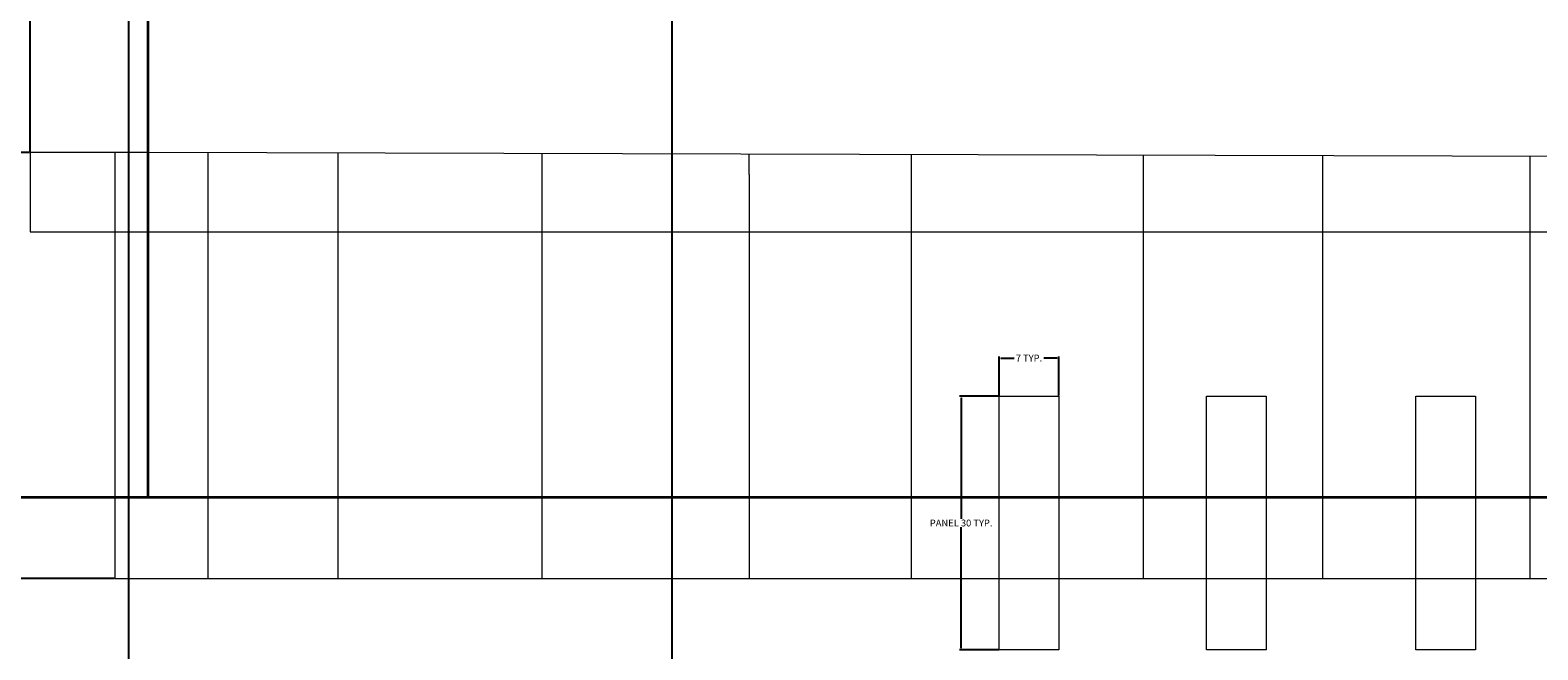
# Model space of a CAD drawing. Units: inches. Extents: x 69 to 650, y -16 to 573.
# Tile 17 of 26: x 205 to 383, y 394 to 467. Entities that reach past the tile are written whole.
import ezdxf

# ---------------------------------------------------------------- set-up
doc = ezdxf.new("R2010")
doc.units = ezdxf.units.IN
doc.header["$MEASUREMENT"] = 0
for name, color, linetype, lineweight in [('A-ANNO-DIMS', 2, 'Continuous', 18), ('A-ELEV', 8, 'Continuous', 18), ('A-WALL', 7, 'Continuous', 35)]:
    doc.layers.add(name, color=color, linetype=linetype, lineweight=lineweight)
doc.styles.get("Standard").update_dxf_attribs({"font": 'arial.ttf'})
doc.dimstyles.get("Standard").update_dxf_attribs({"dimtxt": 0.8125, "dimasz": 0.18, "dimexe": 0.18, "dimexo": 0.0625, "dimgap": 0.09, "dimtad": 0, "dimtih": 1, "dimtoh": 1, "dimdec": 4, "dimzin": 0, "dimdsep": 46, "dimlunit": 4, "dimtxsty": 'Standard', "dimcen": 0.09, "dimadec": 0, "dimazin": 0, "dimtfac": 1, "dimtdec": 4, "dimtofl": 0, "dimtmove": 0, "dimatfit": 3, "dimfxl": 1, "dimtolj": 1, "dimtzin": 0, "dimarcsym": 0})

# ---------------------------------------------------------------- blocks, each defined once
blk = doc.blocks.new('TRIM-VERTICAL-PANEL')
blk.add_lwpolyline([(0, 30.03), (7.06, 30.03), (7.06, 0), (0, 0)], close=True)
blk = doc.blocks.new('*D11')
at = {"layer": 'A-ANNO-DIMS', "color": 0, "lineweight": -2, "transparency": 16777216}
for p, q in [((319.49, 423.88), (314.87, 423.88)), ((315.05, 423.7), (315.05, 409.38)), ((315.05, 394.04), (315.05, 408.37)), ((319.49, 393.86), (314.87, 393.86))]:
    blk.add_line(p, q, dxfattribs=at)
at = {"layer": 'A-ANNO-DIMS', "color": 0, "transparency": 16777216}
for points in [[(315.02, 423.7), (315.08, 423.7), (315.05, 423.88)], [(315.02, 394.04), (315.08, 394.04), (315.05, 393.86)]]:
    blk.add_solid(points, dxfattribs=at)
at = {"layer": 'Defpoints', "color": 0, "transparency": 16777216}
for p in [(315.05, 423.88), (319.55, 423.88), (319.55, 393.86)]:
    blk.add_point(p, dxfattribs=at)
at = {"layer": 'A-ANNO-DIMS', "color": 0, "transparency": 16777216, "insert": (315.05, 408.87), "char_height": 0.8125, "attachment_point": 5}
blk.add_mtext('\\A1;PANEL 30 TYP.', dxfattribs=at)
blk = doc.blocks.new('*D12')
at = {"layer": 'A-ANNO-DIMS', "color": 0, "lineweight": -2, "transparency": 16777216}
for p, q in [((319.55, 423.95), (319.55, 428.57)), ((319.73, 428.39), (321.33, 428.39)), ((326.43, 428.39), (324.83, 428.39)), ((326.61, 423.95), (326.61, 428.57))]:
    blk.add_line(p, q, dxfattribs=at)
at = {"layer": 'A-ANNO-DIMS', "color": 0, "transparency": 16777216}
for points in [[(319.73, 428.42), (319.73, 428.36), (319.55, 428.39)], [(326.43, 428.42), (326.43, 428.36), (326.61, 428.39)]]:
    blk.add_solid(points, dxfattribs=at)
at = {"layer": 'Defpoints', "color": 0, "transparency": 16777216}
for p in [(326.61, 428.39), (319.55, 423.88), (326.61, 423.88)]:
    blk.add_point(p, dxfattribs=at)
at = {"layer": 'A-ANNO-DIMS', "color": 0, "transparency": 16777216, "insert": (323.08, 428.39), "char_height": 0.812, "attachment_point": 5}
blk.add_mtext('\\A1;7 TYP.', dxfattribs=at)
blk = doc.blocks.new('*D19')
at = {"layer": 'A-ANNO-DIMS', "color": 0, "lineweight": -2, "transparency": 16777216}
for p, q in [((99.56, 471.72), (99.56, 572.74)), ((99.74, 572.56), (358.57, 572.56)), ((619.38, 572.56), (360.54, 572.56)), ((619.56, 87.99), (619.56, 572.74))]:
    blk.add_line(p, q, dxfattribs=at)
at = {"layer": 'A-ANNO-DIMS', "color": 0, "transparency": 16777216}
for points in [[(99.74, 572.59), (99.74, 572.53), (99.56, 572.56)], [(619.38, 572.59), (619.38, 572.53), (619.56, 572.56)]]:
    blk.add_solid(points, dxfattribs=at)
at = {"layer": 'Defpoints', "color": 0, "transparency": 16777216}
for p in [(619.56, 572.56), (99.56, 471.66), (619.56, 87.93)]:
    blk.add_point(p, dxfattribs=at)
at = {"layer": 'A-ANNO-DIMS', "color": 0, "transparency": 16777216, "insert": (359.56, 572.56), "char_height": 0.812, "attachment_point": 5}
blk.add_mtext('\\A1;520', dxfattribs=at)
blk = doc.blocks.new('*D45')
at = {"layer": 'A-ANNO-DIMS', "color": 0, "lineweight": -2, "transparency": 16777216}
for p, q in [((216.55, 353.2), (216.55, 572.74)), ((216.73, 572.56), (247.25, 572.56)), ((280.68, 572.56), (250.16, 572.56)), ((280.86, 353.2), (280.86, 572.74))]:
    blk.add_line(p, q, dxfattribs=at)
at = {"layer": 'A-ANNO-DIMS', "color": 0, "transparency": 16777216}
for points in [[(216.73, 572.59), (216.73, 572.53), (216.55, 572.56)], [(280.68, 572.59), (280.68, 572.53), (280.86, 572.56)]]:
    blk.add_solid(points, dxfattribs=at)
at = {"layer": 'Defpoints', "color": 0, "transparency": 16777216}
for p in [(280.86, 572.56), (216.55, 353.14), (280.86, 353.14)]:
    blk.add_point(p, dxfattribs=at)
at = {"layer": 'A-ANNO-DIMS', "color": 0, "transparency": 16777216, "insert": (248.71, 572.56), "char_height": 0.812, "attachment_point": 5}
blk.add_mtext('\\A1;64.32', dxfattribs=at)
blk = doc.blocks.new('*D59')
at = {"layer": 'A-ANNO-DIMS', "color": 0, "lineweight": -2, "transparency": 16777216}
for p, q in [((214.82, 402.3), (70.98, 402.3)), ((71.16, 402.12), (71.16, 394.11)), ((71.16, 385.08), (71.16, 393.1)), ((307.73, 384.9), (70.98, 384.9))]:
    blk.add_line(p, q, dxfattribs=at)
at = {"layer": 'A-ANNO-DIMS', "color": 0, "transparency": 16777216}
for points in [[(71.13, 402.12), (71.19, 402.12), (71.16, 402.3)], [(71.13, 385.08), (71.19, 385.08), (71.16, 384.9)]]:
    blk.add_solid(points, dxfattribs=at)
at = {"layer": 'Defpoints', "color": 0, "transparency": 16777216}
for p in [(71.16, 402.3), (214.89, 402.3), (307.8, 384.9)]:
    blk.add_point(p, dxfattribs=at)
at = {"layer": 'A-ANNO-DIMS', "color": 0, "transparency": 16777216, "insert": (71.16, 393.6), "char_height": 0.812, "attachment_point": 5}
blk.add_mtext('\\A1;17.406', dxfattribs=at)
blk = doc.blocks.new('*D60')
at = {"layer": 'A-ANNO-DIMS', "color": 0, "lineweight": -2, "transparency": 16777216}
for p, q in [((204.8, 452.74), (70.98, 452.74)), ((71.16, 452.56), (71.16, 428.03)), ((71.16, 402.48), (71.16, 427.02)), ((214.82, 402.3), (70.98, 402.3))]:
    blk.add_line(p, q, dxfattribs=at)
at = {"layer": 'A-ANNO-DIMS', "color": 0, "transparency": 16777216}
for points in [[(71.13, 452.56), (71.19, 452.56), (71.16, 452.74)], [(71.13, 402.48), (71.19, 402.48), (71.16, 402.3)]]:
    blk.add_solid(points, dxfattribs=at)
at = {"layer": 'Defpoints', "color": 0, "transparency": 16777216}
for p in [(71.16, 452.74), (204.87, 452.74), (214.89, 402.3)]:
    blk.add_point(p, dxfattribs=at)
at = {"layer": 'A-ANNO-DIMS', "color": 0, "transparency": 16777216, "insert": (71.16, 427.52), "char_height": 0.812, "attachment_point": 5}
blk.add_mtext('\\A1;50.43', dxfattribs=at)
blk = doc.blocks.new('*D62')
at = {"layer": 'A-ANNO-DIMS', "color": 0, "lineweight": -2, "transparency": 16777216}
for p, q in [((204.87, 452.8), (204.87, 572.74)), ((205.05, 572.56), (356.52, 572.56)), ((510.91, 572.56), (359.44, 572.56)), ((511.09, 451.98), (511.09, 572.74))]:
    blk.add_line(p, q, dxfattribs=at)
at = {"layer": 'A-ANNO-DIMS', "color": 0, "transparency": 16777216}
for points in [[(205.05, 572.59), (205.05, 572.53), (204.87, 572.56)], [(510.91, 572.59), (510.91, 572.53), (511.09, 572.56)]]:
    blk.add_solid(points, dxfattribs=at)
at = {"layer": 'Defpoints', "color": 0, "transparency": 16777216}
for p in [(511.09, 572.56), (204.87, 452.74), (511.09, 451.92)]:
    blk.add_point(p, dxfattribs=at)
at = {"layer": 'A-ANNO-DIMS', "color": 0, "transparency": 16777216, "insert": (357.98, 572.56), "char_height": 0.812, "attachment_point": 5}
blk.add_mtext('\\A1;306.2', dxfattribs=at)

msp = doc.modelspace()

# ---------------------------------------------------------------- linework, layer by layer
at = {"layer": 'A-ELEV'}
for p, q in [((218.848, 452.7384), (204.8658, 452.7384)), ((204.8658, 452.7384), (204.8658, 443.3425)), ((214.8863, 452.7384), (214.8863, 402.3042)), ((511.0913, 451.9213), (218.848, 452.7384)), ((225.8833, 452.7187), (225.8833, 402.3042)), ((241.2794, 452.6757), (241.2794, 402.3042)), ((265.4215, 452.6082), (265.4215, 402.3042)), ((289.9685, 450.123), (289.9685, 452.5395)), ((309.1172, 452.486), (309.1172, 402.3042)), ((336.5878, 452.4092), (336.5878, 402.3042)), ((357.8131, 452.3499), (357.8131, 402.3042)), ((382.3703, 452.2812), (382.3703, 402.3042)), ((289.9685, 450.123), (289.9685, 402.3042)), ((204.8658, 443.3425), (511.0913, 443.3425)), ((214.8863, 402.3042), (505.6709, 402.3042))]:
    msp.add_line(p, q, dxfattribs=at)
at = {"layer": 'A-WALL'}
for p, q in [((218.848, 411.93), (218.848, 533.4142)), ((99.556, 411.93), (619.555, 411.93))]:
    msp.add_line(p, q, dxfattribs=at)

# ---------------------------------------------------------------- block references
at = {"layer": 'A-ELEV'}
for p in [(319.551, 393.858), (344.0801, 393.858), (368.8807, 393.858)]:
    msp.add_blockref('TRIM-VERTICAL-PANEL', p, dxfattribs=at)

# ---------------------------------------------------------------- dimensions: what is measured, and where the dimension line sits
at = {"layer": 'A-ANNO-DIMS'}
for base, p1, p2, override, picture, middle in [((619.555, 572.5573), (99.556, 471.6595), (619.555, 87.93), {"dimdec": 0, "dimlfac": 1, "dimrnd": 0, "dimzin": 0, "dimdsep": 46, "dimlunit": 2}, '*D19', (359.5555, 572.5573)), ((511.0913, 572.5573), (204.8658, 452.7384), (511.0913, 451.9213), {"dimdec": 1, "dimlfac": 1, "dimrnd": 0, "dimzin": 0, "dimdsep": 46, "dimlunit": 2}, '*D62', (357.9786, 572.5573)), ((280.864, 572.5573), (216.5473, 353.1381), (280.864, 353.1381), {"dimdec": 2, "dimlfac": 1, "dimrnd": 0, "dimzin": 0, "dimdsep": 46, "dimlunit": 2}, '*D45', (248.7057, 572.5573))]:
    dim = msp.add_linear_dim(base=base, p1=p1, p2=p2, dimstyle='Standard', override=override, dxfattribs=at)
    dim.commit()
    dim.dimension.update_dxf_attribs({"geometry": picture, "text_midpoint": middle})
for base, p1, p2, override, picture, middle in [((71.156, 452.7384), (214.8863, 402.3042), (204.8658, 452.7384), {"dimdec": 2, "dimlfac": 1, "dimrnd": 0, "dimzin": 0, "dimdsep": 46, "dimlunit": 2}, '*D60', (71.156, 427.5213)), ((71.156, 402.3042), (307.7955, 384.8986), (214.8863, 402.3042), {"dimdec": 3, "dimlfac": 1, "dimrnd": 0, "dimzin": 0, "dimdsep": 46, "dimlunit": 2}, '*D59', (71.156, 393.6014))]:
    dim = msp.add_linear_dim(base=base, p1=p1, p2=p2, angle=90, dimstyle='Standard', override=override, dxfattribs=at)
    dim.commit()
    dim.dimension.update_dxf_attribs({"geometry": picture, "text_midpoint": middle})
dim = msp.add_linear_dim(base=(326.6113, 428.3879), p1=(319.5513, 423.8839), p2=(326.6113, 423.8839), text='<> TYP.', dimstyle='Standard', override={"dimdec": 0, "dimlfac": 1, "dimrnd": 0, "dimzin": 0, "dimdsep": 46, "dimlunit": 2}, dxfattribs=at)
dim.commit()
dim.dimension.update_dxf_attribs({"geometry": '*D12', "text_midpoint": (323.0813, 428.3879)})
dim = msp.add_linear_dim(base=(315.0474, 423.8839), p1=(319.5513, 393.8576), p2=(319.5513, 423.8839), angle=90, text='PANEL <> TYP.', dimstyle='Standard', override={"dimdec": 0, "dimlfac": 1, "dimrnd": 0, "dimzin": 0, "dimdsep": 46, "dimlunit": 2}, dxfattribs=at)
dim.commit()
dim.dimension.update_dxf_attribs({"geometry": '*D11', "text_midpoint": (315.0474, 408.8708)})

doc.saveas('drawing.dxf')
